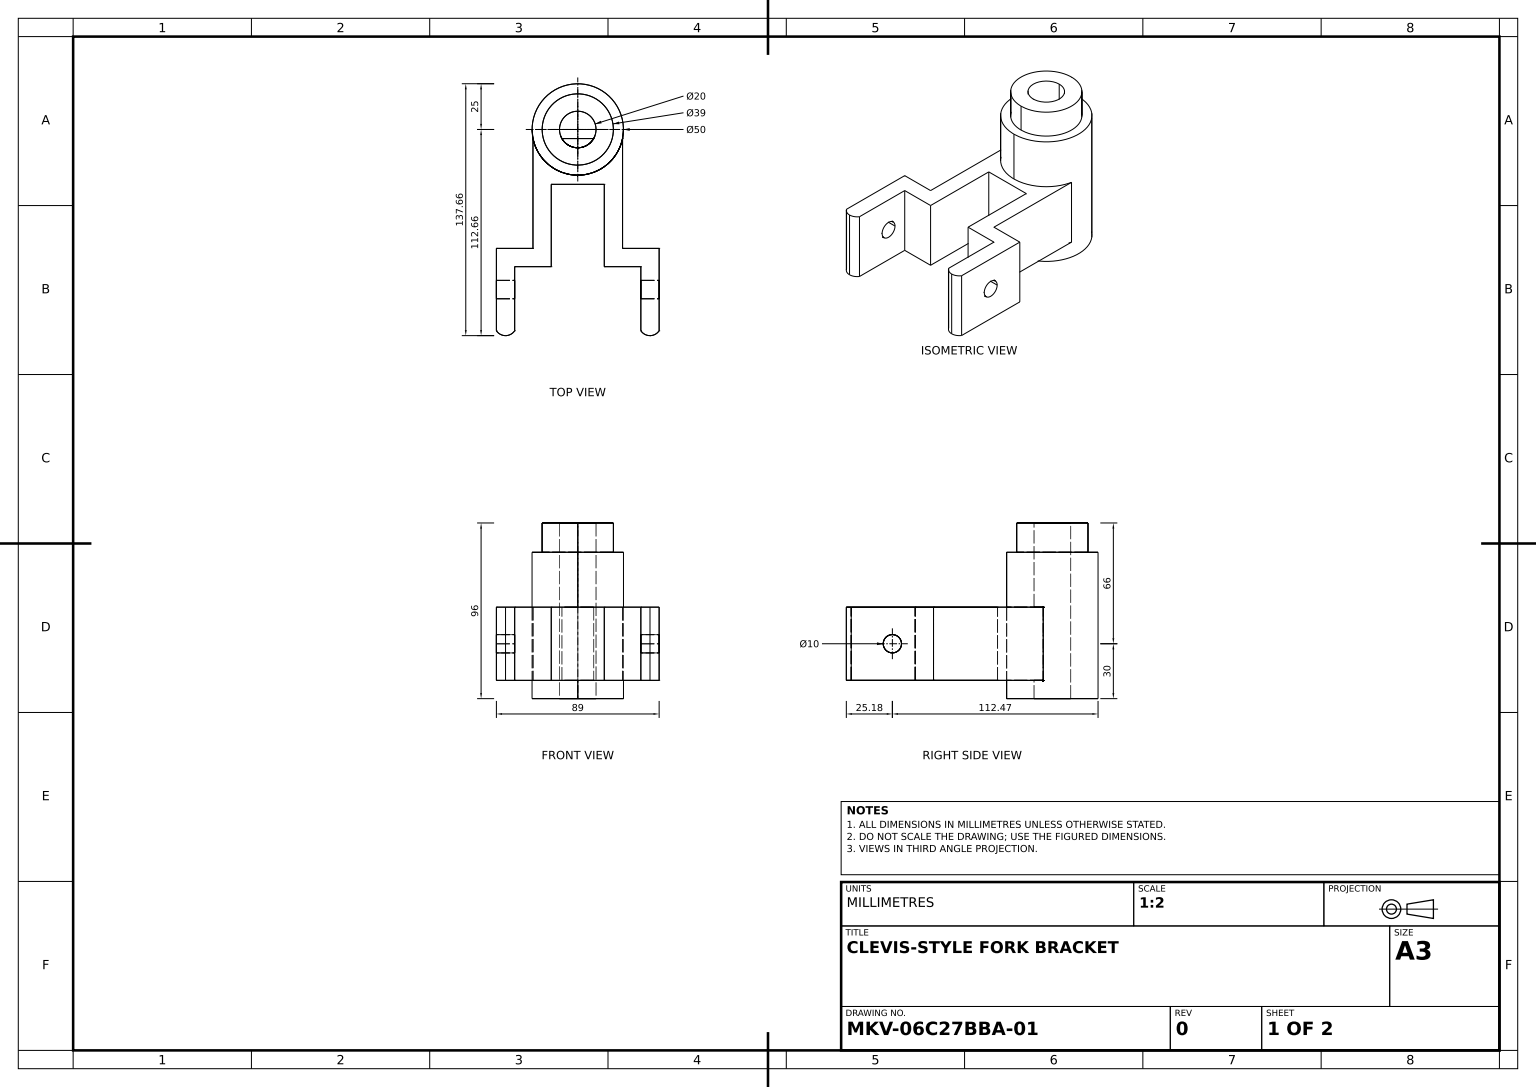
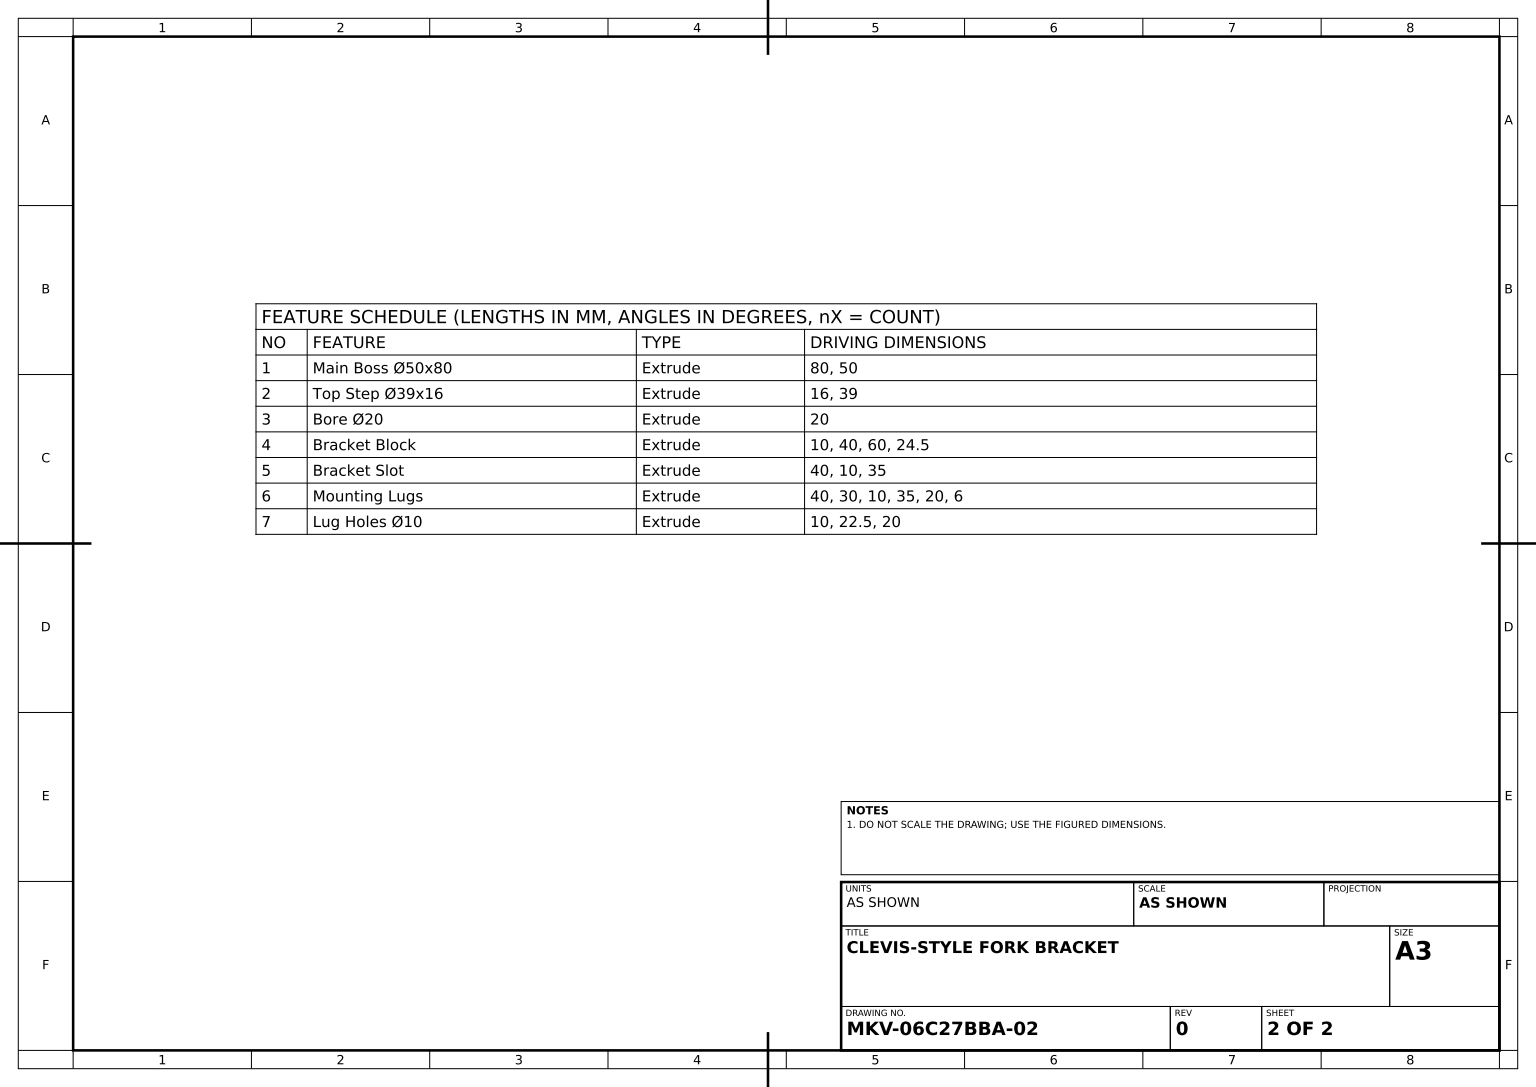
SolidWorks part; units mm, degrees
material "Plain Carbon Steel"
ref_plane "Front Plane" through (0, 0, 0) normal (0, 0, 1) x (1, 0, 0)
ref_plane "Top Plane" through (0, 0, 0) normal (0, 1, 0) x (1, 0, 0)
ref_plane "Right Plane" through (0, 0, 0) normal (1, 0, 0) x (0, 0, -1)
sketch "Main Boss Sketch Ø50" plane through (0, 0, 0) normal (0, 1, 0) x (1, 0, 0)
  circle A0 centre (0, 0) radius 25
  dimension "D1" = 50
extrude "Main Boss Ø50x80" add sketch "Main Boss Sketch Ø50" along normal blind 80
sketch "Top Step Sketch Ø39" plane through (0, 80, 0) normal (0, 1, 0) x (1, 0, 0)
  circle A0 centre (0, 0) radius 19.5
  dimension "D1" = 39
extrude "Top Step Ø39x16" add sketch "Top Step Sketch Ø39" along normal blind 16
sketch "Bore Sketch Ø20" plane through (0, 96, 0) normal (0, 1, 0) x (1, 0, 0)
  circle A0 centre (0, 0) radius 10
  dimension "D1" = 20
extrude "Bore Ø20" cut sketch "Bore Sketch Ø20" against normal through all
ref_plane "Bracket Plane Offset 10" through (0, 10, 0) normal (0, 1, 0) x (1, 0, 0)
sketch "Bracket Block Sketch" plane through (0, 10, 0) normal (0, 1, 0) x (1, 0, 0)
  line L1 (-24.5, -4.9749) -> (24.5, -4.9749)
  line L2 (-24.5, -4.9749) -> (-24.5, -64.9749)
  line L3 (-24.5, -64.9749) -> (24.5, -64.9749)
  line L4 (24.5, -4.9749) -> (24.5, -64.9749)
  circle A0 centre (0, 0) radius 25 construction
  dimension "D1" = 60
  dimension "D2" = 24.5
  dimension "D3" = 24.5
extrude "Bracket Block" add sketch "Bracket Block Sketch" along normal blind 40
sketch "Bracket Slot Sketch" plane through (0, 50, 0) normal (0, 1, 0) x (1, 0, 0)
  line L0 (-24.5, -64.9749) -> (24.5, -64.9749) construction
  line L1 (-14.5, -64.9749) -> (14.5, -64.9749)
  line L2 (-14.5, -64.9749) -> (-14.5, -29.9749)
  line L3 (-14.5, -29.9749) -> (14.5, -29.9749)
  line L4 (14.5, -64.9749) -> (14.5, -29.9749)
  dimension "D1" = 10
  dimension "D2" = 10
  dimension "D3" = 35
extrude "Bracket Slot" cut sketch "Bracket Slot Sketch" against normal blind 40
sketch "Mounting Lugs Sketch" plane through (0, 50, 0) normal (0, 1, 0) x (1, 0, 0)
  line L1 (14.5, -64.9749) -> (44.5, -64.9749)
  line L2 (14.5, -64.9749) -> (14.5, -74.9749)
  line L3 (14.5, -74.9749) -> (34.5, -74.9749)
  line L4 (44.5, -64.9749) -> (44.5, -74.9749)
  line L6 (44.5, -74.9749) -> (44.5, -109.9749)
  line L8 (34.5, -74.9749) -> (34.5, -109.9749)
  line L9 (-14.5, -64.9749) -> (-44.5, -64.9749)
  line L10 (-14.5, -64.9749) -> (-14.5, -74.9749)
  line L11 (-14.5, -74.9749) -> (-34.5, -74.9749)
  line L12 (-44.5, -64.9749) -> (-44.5, -74.9749)
  line L14 (-44.5, -74.9749) -> (-44.5, -109.9749)
  line L16 (-34.5, -74.9749) -> (-34.5, -109.9749)
  arc A0 (-44.5, -109.9749) -> (-34.5, -109.9749) centre (-39.5, -106.6583) ccw
  arc A1 (34.5, -109.9749) -> (44.5, -109.9749) centre (39.5, -106.6583) ccw
  dimension "D11" = 6
  dimension "D12" = 6
  dimension "D1" = 30
  dimension "D2" = 10
  dimension "D3" = 10
  dimension "D4" = 35
  dimension "D5" = 20
  dimension "D6" = 30
  dimension "D7" = 10
  dimension "D8" = 10
  dimension "D9" = 35
  dimension "D10" = 35
  dimension "D13" = 10
  dimension "D14" = 35
extrude "Mounting Lugs" add sketch "Mounting Lugs Sketch" against normal blind 40
sketch "Lug Hole Sketch Ø10" plane through (44.5, 0, 0) normal (1, 0, 0) x (0, 0, -1)
  line L0 (-109.9749, 50) -> (-64.9749, 50) construction
  circle A0 centre (-87.4749, 30) radius 5
  dimension "D1" = 10
  dimension "D2" = 22.5
  dimension "D3" = 20
extrude "Lug Holes Ø10" cut sketch "Lug Hole Sketch Ø10" against normal through all
